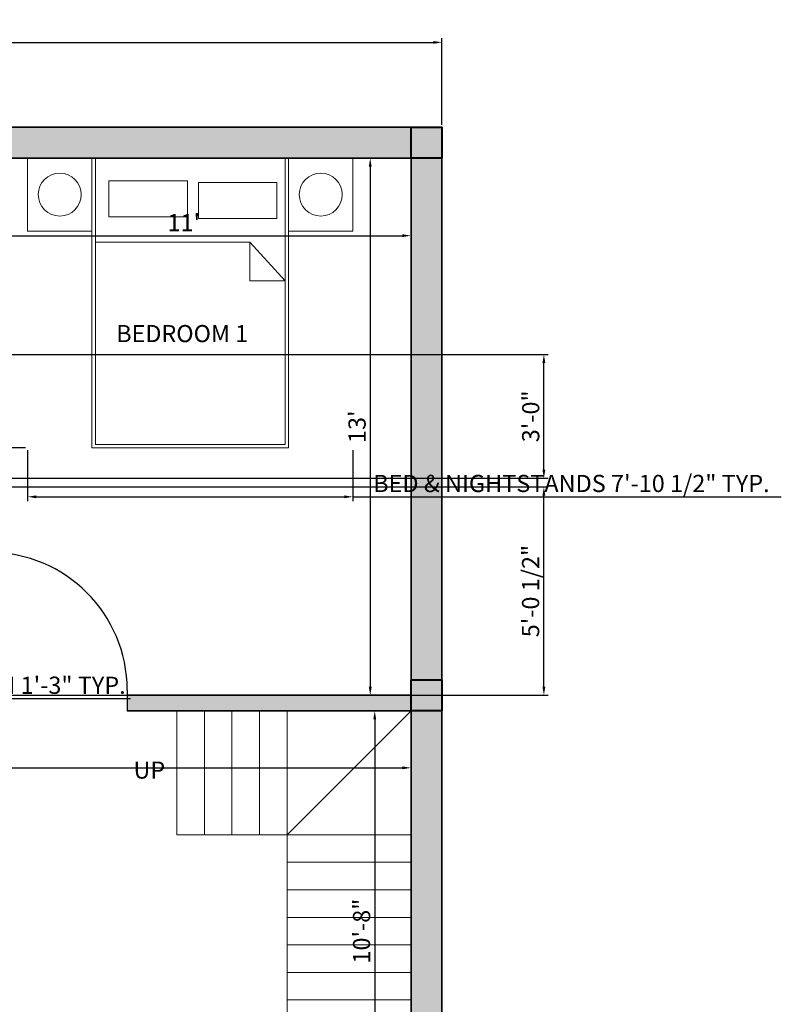
# Model space of a CAD drawing. Units: inches. Extents: x 1674 to 2231, y 1328 to 1959.
# Tile 6 of 6: x 2010 to 2231, y 1664 to 1950. Entities that reach past the tile are written whole.
import ezdxf

# ---------------------------------------------------------------- set-up
doc = ezdxf.new("R2010")
doc.units = ezdxf.units.IN
for name, color, linetype, lineweight in [('A-ANNO-DIMS', 113, 'Continuous', 18), ('A-ANNO-TEXT', 113, 'Continuous', 18), ('A-AREA-IDEN', 113, 'Continuous', 18), ('A-COLS-PATT', 10, 'Continuous', 13), ('A-FLOR-STRS', 7, 'Continuous', 18), ('A-WALL-PATT', 140, 'Continuous', 13), ('COLUMN', 10, 'Continuous', 40), ('DOOR', 54, 'Continuous', 25), ('FUR', 211, 'Continuous', 18), ('WALL', 7, 'Continuous', 35)]:
    doc.layers.add(name, color=color, linetype=linetype, lineweight=lineweight)
doc.styles.get("Standard").update_dxf_attribs({"font": 'arial.ttf'})
doc.dimstyles.new('ISO-25', dxfattribs={"dimtxt": 5, "dimasz": 2.5, "dimexe": 1.25, "dimexo": 0.625, "dimtad": 1, "dimdec": 0, "dimlunit": 4, "dimtxsty": 'Standard', "dimcen": 2.5, "dimadec": 0, "dimazin": 0, "dimtfac": 1, "dimtdec": 0, "dimtmove": 0, "dimatfit": 3, "dimfxl": 1, "dimarcsym": 0})

# ---------------------------------------------------------------- blocks, each defined once
blk = doc.blocks.new('*U2')
for p, q in [((0, 0), (0, -6)), ((40, 0), (40, -6))]:
    blk.add_line(p, q)
blk.add_lwpolyline([(0, 0), (0, 40), (1.75, 40), (1.75, 0)], close=True)
blk.add_arc((0, 0), 40, 0, 90)
blk = doc.blocks.new('*D9')
at = {"layer": 'A-ANNO-DIMS', "color": 0, "lineweight": -2, "transparency": 16777216}
for p, q in [((1736.27, 1918.98), (1736.27, 1944.21)), ((1738.77, 1942.96), (2129.77, 1942.96)), ((2132.27, 1918.98), (2132.27, 1944.21))]:
    blk.add_line(p, q, dxfattribs=at)
at = {"layer": 'A-ANNO-DIMS', "color": 0, "lineweight": 100, "transparency": 16777216}
for points in [[(1738.77, 1943.37), (1738.77, 1942.54), (1736.27, 1942.96)], [(2129.77, 1943.37), (2129.77, 1942.54), (2132.27, 1942.96)]]:
    blk.add_solid(points, dxfattribs=at)
at = {"layer": 'Defpoints', "color": 0, "lineweight": 100, "transparency": 16777216}
for p in [(2132.27, 1942.96), (1736.27, 1918.36), (2132.27, 1918.36)]:
    blk.add_point(p, dxfattribs=at)
at = {"layer": 'A-ANNO-DIMS', "color": 0, "transparency": 16777216, "insert": (1934.27, 1946.13), "char_height": 5, "attachment_point": 5}
blk.add_mtext("33'", dxfattribs=at)
blk = doc.blocks.new('*D19')
at = {"layer": 'A-ANNO-DIMS', "color": 0, "lineweight": -2, "transparency": 16777216}
for p, q in [((1991.27, 1908.73), (1991.27, 1885.57)), ((2123.27, 1908.73), (2123.27, 1885.57)), ((1993.77, 1886.82), (2120.77, 1886.82))]:
    blk.add_line(p, q, dxfattribs=at)
at = {"layer": 'A-ANNO-DIMS', "color": 0, "lineweight": 100, "transparency": 16777216}
for points in [[(1993.77, 1887.24), (1993.77, 1886.4), (1991.27, 1886.82)], [(2120.77, 1887.24), (2120.77, 1886.4), (2123.27, 1886.82)]]:
    blk.add_solid(points, dxfattribs=at)
at = {"layer": 'Defpoints', "color": 0, "lineweight": 100, "transparency": 16777216}
for p in [(1991.27, 1909.36), (2123.27, 1909.36), (2123.27, 1886.82)]:
    blk.add_point(p, dxfattribs=at)
at = {"layer": 'A-ANNO-DIMS', "color": 0, "transparency": 16777216, "insert": (2057.27, 1889.95), "char_height": 5, "attachment_point": 5}
blk.add_mtext("11'", dxfattribs=at)
blk = doc.blocks.new('*D20')
at = {"layer": 'A-ANNO-DIMS', "color": 0, "lineweight": -2, "transparency": 16777216}
for p, q in [((2122.65, 1909.36), (2110.18, 1909.36)), ((2111.43, 1906.86), (2111.43, 1755.81)), ((2122.65, 1753.31), (2110.18, 1753.31))]:
    blk.add_line(p, q, dxfattribs=at)
at = {"layer": 'A-ANNO-DIMS', "color": 0, "lineweight": 100, "transparency": 16777216}
for points in [[(2111.01, 1906.86), (2111.85, 1906.86), (2111.43, 1909.36)], [(2111.01, 1755.81), (2111.85, 1755.81), (2111.43, 1753.31)]]:
    blk.add_solid(points, dxfattribs=at)
at = {"layer": 'Defpoints', "color": 0, "lineweight": 100, "transparency": 16777216}
for p in [(2123.27, 1909.36), (2111.43, 1753.31), (2123.27, 1753.31)]:
    blk.add_point(p, dxfattribs=at)
at = {"layer": 'A-ANNO-DIMS', "color": 0, "transparency": 16777216, "insert": (2108.25, 1831.33), "char_height": 5, "attachment_point": 5, "rotation": 90}
blk.add_mtext("13'", dxfattribs=at)
blk = doc.blocks.new('*D21')
at = {"layer": 'A-ANNO-DIMS', "color": 0, "lineweight": -2, "transparency": 16777216}
for p, q in [((2122.65, 1748.86), (2111.49, 1748.86)), ((2112.74, 1746.36), (2112.74, 1623.36)), ((2122.65, 1620.86), (2111.49, 1620.86))]:
    blk.add_line(p, q, dxfattribs=at)
at = {"layer": 'A-ANNO-DIMS', "color": 0, "lineweight": 100, "transparency": 16777216}
for points in [[(2112.32, 1746.36), (2113.15, 1746.36), (2112.74, 1748.86)], [(2112.32, 1623.36), (2113.15, 1623.36), (2112.74, 1620.86)]]:
    blk.add_solid(points, dxfattribs=at)
at = {"layer": 'Defpoints', "color": 0, "lineweight": 100, "transparency": 16777216}
for p in [(2123.27, 1748.86), (2112.74, 1620.86), (2123.27, 1620.86)]:
    blk.add_point(p, dxfattribs=at)
at = {"layer": 'A-ANNO-DIMS', "color": 0, "transparency": 16777216, "insert": (2109.56, 1684.86), "char_height": 5, "attachment_point": 5, "rotation": 90}
blk.add_mtext('10\'-8"', dxfattribs=at)
blk = doc.blocks.new('*D33')
at = {"layer": 'A-ANNO-DIMS', "color": 0, "lineweight": -2, "transparency": 16777216}
for p, q in [((1821.77, 1748.23), (1821.77, 1731.03)), ((2123.27, 1748.18), (2123.27, 1731.03)), ((1824.27, 1732.28), (2120.77, 1732.28))]:
    blk.add_line(p, q, dxfattribs=at)
at = {"layer": 'A-ANNO-DIMS', "color": 0, "lineweight": 100, "transparency": 16777216}
for points in [[(1824.27, 1732.69), (1824.27, 1731.86), (1821.77, 1732.28)], [(2120.77, 1732.69), (2120.77, 1731.86), (2123.27, 1732.28)]]:
    blk.add_solid(points, dxfattribs=at)
at = {"layer": 'Defpoints', "color": 0, "lineweight": 100, "transparency": 16777216}
for p in [(1821.77, 1748.86), (2123.27, 1748.81), (2123.27, 1732.28)]:
    blk.add_point(p, dxfattribs=at)
at = {"layer": 'A-ANNO-DIMS', "color": 0, "transparency": 16777216, "insert": (1972.52, 1735.45), "char_height": 5, "attachment_point": 5}
blk.add_mtext('25\'-2"', dxfattribs=at)
blk = doc.blocks.new('BED-DOUBLE-WITH-NIGHTSTANDS')
for p, q in [((35.61, 74.81), (24.38, 64.59)), ((35.61, 64.59), (35.61, 74.81)), ((24.38, 19.67), (24.38, 64.59)), ((24.38, 64.59), (35.61, 64.59))]:
    blk.add_line(p, q)
for points in [[(0, 75.81), (21.22, 75.81), (21.22, 94.48), (0, 94.48)], [(0, 19.67), (83.2, 19.67), (83.2, 74.81), (0, 74.81)], [(7.05, 49.62), (17.52, 49.62), (17.52, 72.41), (7.05, 72.41)], [(6.58, 23.6), (17.06, 23.6), (17.06, 46.39), (6.58, 46.39)], [(0, 0), (21.22, 0), (21.22, 18.67), (0, 18.67)]]:
    blk.add_lwpolyline(points, close=True)
blk.add_lwpolyline([(0, 18.67), (84.2, 18.67), (84.2, 75.81), (0, 75.81)])
for centre in [(10.61, 85.15), (10.61, 9.33)]:
    blk.add_circle(centre, 6.24)
blk = doc.blocks.new('*D42')
at = {"layer": 'A-ANNO-DIMS', "color": 0, "lineweight": -2, "transparency": 16777216}
for p, q in [((1969.88, 1754.02), (1969.88, 1751.15)), ((1984.85, 1754.02), (1984.85, 1751.15)), ((1972.38, 1752.4), (1982.35, 1752.4)), ((1984.85, 1752.4), (2041.76, 1752.4))]:
    blk.add_line(p, q, dxfattribs=at)
at = {"layer": 'A-ANNO-DIMS', "color": 0, "lineweight": 100, "transparency": 16777216}
for points in [[(1972.38, 1752.81), (1972.38, 1751.98), (1969.88, 1752.4)], [(1982.35, 1752.81), (1982.35, 1751.98), (1984.85, 1752.4)]]:
    blk.add_solid(points, dxfattribs=at)
at = {"layer": 'Defpoints', "color": 0, "lineweight": 100, "transparency": 16777216}
for p in [(1969.88, 1754.64), (1984.85, 1754.64), (1984.85, 1752.4)]:
    blk.add_point(p, dxfattribs=at)
at = {"layer": 'A-ANNO-DIMS', "color": 0, "transparency": 16777216, "insert": (2014.56, 1755.61), "char_height": 5, "attachment_point": 5}
blk.add_mtext('BASIN 1\'-3" TYP.', dxfattribs=at)
blk = doc.blocks.new('*D46')
at = {"layer": 'A-ANNO-DIMS', "color": 0, "lineweight": -2, "transparency": 16777216}
for p, q in [((2011.91, 1824.53), (2011.91, 1809.74)), ((2106.39, 1824.53), (2106.39, 1809.74)), ((2014.41, 1810.99), (2103.89, 1810.99)), ((2106.39, 1810.99), (2230.84, 1810.99))]:
    blk.add_line(p, q, dxfattribs=at)
at = {"layer": 'A-ANNO-DIMS', "color": 0, "lineweight": 100, "transparency": 16777216}
for points in [[(2014.41, 1811.4), (2014.41, 1810.57), (2011.91, 1810.99)], [(2103.89, 1811.4), (2103.89, 1810.57), (2106.39, 1810.99)]]:
    blk.add_solid(points, dxfattribs=at)
at = {"layer": 'Defpoints', "color": 0, "lineweight": 100, "transparency": 16777216}
for p in [(2011.91, 1825.16), (2106.39, 1825.16), (2106.39, 1810.99)]:
    blk.add_point(p, dxfattribs=at)
at = {"layer": 'A-ANNO-DIMS', "color": 0, "transparency": 16777216, "insert": (2169.86, 1814.21), "char_height": 5, "attachment_point": 5}
blk.add_mtext('BED & NIGHTSTANDS 7\'-10 1/2" TYP.', dxfattribs=at)
blk = doc.blocks.new('*D47')
at = {"layer": 'A-ANNO-DIMS', "color": 0, "lineweight": -2, "transparency": 16777216}
for p, q in [((2011.29, 1909.36), (1996.49, 1909.36)), ((1997.74, 1906.86), (1997.74, 1827.66)), ((2011.29, 1825.16), (1996.49, 1825.16))]:
    blk.add_line(p, q, dxfattribs=at)
at = {"layer": 'A-ANNO-DIMS', "color": 0, "lineweight": 100, "transparency": 16777216}
for points in [[(1997.32, 1906.86), (1998.16, 1906.86), (1997.74, 1909.36)], [(1997.32, 1827.66), (1998.16, 1827.66), (1997.74, 1825.16)]]:
    blk.add_solid(points, dxfattribs=at)
at = {"layer": 'Defpoints', "color": 0, "lineweight": 100, "transparency": 16777216}
for p in [(2011.91, 1909.36), (1997.74, 1825.16), (2011.91, 1825.16)]:
    blk.add_point(p, dxfattribs=at)
at = {"layer": 'A-ANNO-DIMS', "color": 0, "transparency": 16777216, "insert": (1994.56, 1867.26), "char_height": 5, "attachment_point": 5, "rotation": 90}
blk.add_mtext('7\'-0" TYP.', dxfattribs=at)
blk = doc.blocks.new('*D52')
at = {"layer": 'A-ANNO-DIMS', "color": 0, "lineweight": -2, "transparency": 16777216}
for p, q in [((1987.4, 1813.86), (2163.12, 1813.86)), ((2161.87, 1755.86), (2161.87, 1811.36)), ((1987.4, 1753.36), (2163.12, 1753.36))]:
    blk.add_line(p, q, dxfattribs=at)
at = {"layer": 'A-ANNO-DIMS', "color": 0, "lineweight": 100, "transparency": 16777216}
for points in [[(2161.45, 1811.36), (2162.29, 1811.36), (2161.87, 1813.86)], [(2161.45, 1755.86), (2162.29, 1755.86), (2161.87, 1753.36)]]:
    blk.add_solid(points, dxfattribs=at)
at = {"layer": 'Defpoints', "color": 0, "lineweight": 100, "transparency": 16777216}
for p in [(1986.77, 1813.86), (2161.87, 1813.86), (1986.77, 1753.36)]:
    blk.add_point(p, dxfattribs=at)
at = {"layer": 'A-ANNO-DIMS', "color": 0, "transparency": 16777216, "insert": (2158.66, 1783.61), "char_height": 5, "attachment_point": 5, "rotation": 90}
blk.add_mtext('5\'-0 1/2"', dxfattribs=at)
blk = doc.blocks.new('*D53')
at = {"layer": 'A-ANNO-DIMS', "color": 0, "lineweight": -2, "transparency": 16777216}
for p, q in [((1987.4, 1852.36), (2163.12, 1852.36)), ((2161.87, 1818.86), (2161.87, 1849.86)), ((1987.4, 1816.36), (2163.12, 1816.36))]:
    blk.add_line(p, q, dxfattribs=at)
at = {"layer": 'A-ANNO-DIMS', "color": 0, "lineweight": 100, "transparency": 16777216}
for points in [[(2161.45, 1849.86), (2162.29, 1849.86), (2161.87, 1852.36)], [(2161.45, 1818.86), (2162.29, 1818.86), (2161.87, 1816.36)]]:
    blk.add_solid(points, dxfattribs=at)
at = {"layer": 'Defpoints', "color": 0, "lineweight": 100, "transparency": 16777216}
for p in [(1986.77, 1852.36), (2161.87, 1852.36), (1986.77, 1816.36)]:
    blk.add_point(p, dxfattribs=at)
at = {"layer": 'A-ANNO-DIMS', "color": 0, "transparency": 16777216, "insert": (2158.69, 1834.36), "char_height": 5, "attachment_point": 5, "rotation": 90}
blk.add_mtext('3\'-0"', dxfattribs=at)

msp = doc.modelspace()

# ---------------------------------------------------------------- hatches: boundary and pattern name
at = {"layer": 'A-COLS-PATT'}
h = msp.add_hatch(color=256, dxfattribs=at)
h.dxf.hatch_style = 1
h.paths.add_polyline_path([(1745.27, 1918.36), (1736.27, 1918.36), (1736.27, 1909.36), (1745.27, 1909.36)])
h.paths.add_polyline_path([(1886.27, 1918.36), (1877.27, 1918.36), (1877.27, 1909.36), (1886.27, 1909.36)])
h.paths.add_polyline_path([(1995.77, 1918.36), (1986.77, 1918.36), (1986.77, 1909.36), (1995.77, 1909.36)])
h.paths.add_polyline_path([(2132.27, 1918.36), (2123.27, 1918.36), (2123.27, 1909.36), (2132.27, 1909.36)])
h.paths.add_polyline_path([(1745.27, 1757.86), (1736.27, 1757.86), (1736.27, 1748.86), (1745.27, 1748.86)])
h.paths.add_polyline_path([(1886.27, 1757.86), (1877.27, 1757.86), (1877.27, 1748.86), (1886.27, 1748.86)])
h.paths.add_polyline_path([(2132.27, 1757.81), (2123.27, 1757.81), (2123.27, 1748.81), (2132.27, 1748.81)])
h.paths.add_polyline_path([(1995.77, 1757.86), (1986.77, 1757.86), (1986.77, 1748.86), (1995.77, 1748.86)])
h.paths.add_polyline_path([(2132.27, 1625.36), (2123.27, 1625.36), (2123.27, 1616.36), (2132.27, 1616.36)])
h.paths.add_polyline_path([(1995.77, 1625.36), (1986.77, 1625.36), (1986.77, 1616.36), (1995.77, 1616.36)])
h.paths.add_polyline_path([(1869.77, 1604.86), (1860.77, 1604.86), (1860.77, 1595.86), (1869.77, 1595.86)])
h.paths.add_polyline_path([(1745.27, 1609.36), (1736.27, 1609.36), (1736.27, 1600.36), (1745.27, 1600.36)])
h.paths.add_polyline_path([(1745.27, 1504.36), (1736.27, 1504.36), (1736.27, 1495.36), (1745.27, 1495.36)])
h.paths.add_polyline_path([(1870.95, 1504.36), (1861.95, 1504.36), (1861.95, 1495.36), (1870.95, 1495.36)])
h.paths.add_polyline_path([(1995.77, 1504.36), (1986.77, 1504.36), (1986.77, 1495.36), (1995.77, 1495.36)])
h.paths.add_polyline_path([(1995.77, 1447.36), (1986.77, 1447.36), (1986.77, 1438.36), (1995.77, 1438.36)])
h.paths.add_polyline_path([(2132.27, 1447.36), (2123.27, 1447.36), (2123.27, 1438.36), (2132.27, 1438.36)])
at = {"layer": 'A-WALL-PATT'}
h = msp.add_hatch(color=256, dxfattribs=at)
h.dxf.hatch_style = 1
h.paths.add_polyline_path([(1877.27, 1918.36), (1745.27, 1918.36), (1745.27, 1909.36), (1877.27, 1909.36)])
h.paths.add_polyline_path([(1986.77, 1918.36), (1886.27, 1918.36), (1886.27, 1909.36), (1986.77, 1909.36)])
h.paths.add_polyline_path([(2123.27, 1918.36), (1995.77, 1918.36), (1995.77, 1909.36), (2123.27, 1909.36)])
h.paths.add_polyline_path([(1894.11, 1861.36), (1886.27, 1861.36), (1886.27, 1865.74), (1881.77, 1865.74), (1881.77, 1808), (1881.77, 1798.89), (1884.87, 1798.89, -0.017002), (1886.27, 1798.84), (1886.27, 1852.36), (1894.11, 1852.36)])
h.paths.add_polyline_path([(1952.87, 1861.36), (1919.24, 1861.36), (1919.24, 1852.36), (1952.87, 1852.36)])
h.paths.add_polyline_path([(1991.27, 1865.74), (1986.77, 1865.74), (1986.77, 1861.36), (1976.26, 1861.36), (1976.26, 1852.36), (1986.77, 1852.36), (1986.77, 1847.49), (1986.77, 1757.86), (1991.27, 1757.86), (1991.27, 1852.36)])
h.paths.add_polyline_path([(1986.77, 1816.36), (1938.77, 1816.36), (1938.77, 1813.86), (1986.77, 1813.86)])
h.paths.add_polyline_path([(1934.27, 1819.36), (1886.27, 1819.36), (1886.27, 1816.86), (1934.27, 1816.86)])
h.paths.add_polyline_path([(1938.77, 1852.36), (1934.27, 1852.36), (1934.27, 1753.36), (1934.27, 1748.86), (1938.77, 1748.86), (1938.77, 1753.36)])
h.paths.add_polyline_path([(1934.27, 1777.36), (1915.46, 1777.36), (1886.27, 1777.36), (1886.27, 1772.86), (1934.27, 1772.86)])
h.paths.add_polyline_path([(1986.77, 1753.36), (1967.96, 1753.36), (1961.77, 1753.36, -0.017002), (1961.81, 1751.95), (1961.81, 1748.86), (1986.77, 1748.86)])
h.paths.add_polyline_path([(2000.84, 1753.36), (1995.77, 1753.36), (1995.77, 1748.86), (2000.84, 1748.86)])
h.paths.add_polyline_path([(1941.17, 1751.95), (1941.17, 1753.36), (1938.77, 1753.36), (1938.77, 1748.86), (1941.17, 1748.86)])
h.paths.add_polyline_path([(1877.27, 1753.36), (1875.49, 1753.36), (1875.49, 1748.86), (1877.27, 1748.86)])
h.paths.add_polyline_path([(1745.27, 1909.36), (1736.27, 1909.36), (1736.27, 1757.86), (1745.27, 1757.86), (1745.27, 1773.01)])
h.paths.add_polyline_path([(1778.41, 1645.36), (1745.27, 1645.36), (1745.27, 1640.86), (1778.41, 1640.86)])
h.paths.add_polyline_path([(1821.77, 1645.36), (1821.77, 1668.45), (1817.27, 1668.45), (1817.27, 1645.36), (1817.27, 1640.86), (1821.77, 1640.86)])
h.paths.add_polyline_path([(1817.27, 1645.36), (1813.39, 1645.36), (1813.39, 1640.86), (1817.27, 1640.86)])
h.paths.add_polyline_path([(1821.77, 1640.86), (1817.27, 1640.86), (1817.27, 1604.86), (1817.27, 1600.36), (1821.77, 1600.36)])
h.paths.add_polyline_path([(1825.14, 1604.86), (1821.77, 1604.86), (1821.77, 1600.36), (1825.14, 1600.36)])
h.paths.add_polyline_path([(1781.27, 1604.86), (1745.27, 1604.86), (1745.27, 1600.36), (1781.27, 1600.36)])
h = msp.add_hatch(color=256, dxfattribs=at)
h.dxf.hatch_style = 1
h.paths.add_polyline_path([(2132.27, 1909.36), (2123.27, 1909.36), (2123.27, 1757.81), (2132.27, 1757.81)], flags=17)
h.paths.add_polyline_path([(2123.27, 1753.36), (2040.84, 1753.36), (2040.84, 1748.86), (2123.27, 1748.86)], flags=17)
h.paths.add_polyline_path([(1840.51, 1753.36), (1745.27, 1753.36), (1745.27, 1748.86), (1817.27, 1748.86), (1840.51, 1748.86)], flags=17)
h.paths.add_polyline_path([(1745.27, 1748.86), (1736.27, 1748.86), (1736.27, 1609.36), (1745.27, 1609.36), (1745.27, 1640.86)], flags=17)
h.paths.add_polyline_path([(1745.27, 1600.36), (1736.27, 1600.36), (1736.27, 1504.36), (1745.27, 1504.36)], flags=17)
h.paths.add_polyline_path([(1745.27, 1495.36), (1736.27, 1495.36), (1736.27, 1447.36), (1745.27, 1447.36)], flags=17)
h.paths.add_polyline_path([(1820.35, 1504.36), (1787.69, 1504.36), (1787.69, 1495.36), (1820.35, 1495.36)], flags=17)
h.paths.add_polyline_path([(1750.58, 1504.36), (1745.27, 1504.36), (1745.27, 1495.36), (1750.58, 1495.36)], flags=17)
h.paths.add_polyline_path([(1861.95, 1504.36), (1857.47, 1504.36), (1857.47, 1495.36), (1861.95, 1495.36)], flags=17)
h.paths.add_polyline_path([(1873.66, 1504.36), (1870.95, 1504.36), (1870.95, 1495.36), (1873.66, 1495.36)], flags=17)
h.paths.add_polyline_path([(1900.85, 1501.36), (1900.85, 1504.36), (1895.88, 1504.36), (1895.88, 1495.36), (1900.85, 1495.36)], flags=17)
h.paths.add_polyline_path([(1869.77, 1595.86), (1865.27, 1595.86), (1865.27, 1504.36), (1869.77, 1504.36)], flags=17)
h.paths.add_polyline_path([(1958.26, 1504.36), (1940.74, 1504.36, -0.01877), (1940.85, 1501.36), (1940.85, 1495.36), (1958.26, 1495.36)], flags=17)
h.paths.add_polyline_path([(1995.77, 1531.51), (1986.77, 1531.51), (1986.77, 1504.36), (1995.77, 1504.36)], flags=17)
h.paths.add_polyline_path([(1986.77, 1504.36), (1980.49, 1504.36), (1980.49, 1495.36), (1986.77, 1495.36)], flags=17)
h.paths.add_polyline_path([(1995.77, 1616.36), (1986.77, 1616.36), (1986.77, 1585.02), (1995.77, 1585.02)], flags=17)
h.paths.add_polyline_path([(2000.1, 1620.86), (1995.77, 1620.86), (1995.77, 1616.36), (2000.1, 1616.36)], flags=17)
h.paths.add_polyline_path([(2053.57, 1620.86), (2040.1, 1620.86), (2040.1, 1616.36), (2053.57, 1616.36)], flags=17)
h.paths.add_polyline_path([(2123.27, 1620.86), (2109.12, 1620.86), (2109.12, 1616.36), (2123.27, 1616.36)], flags=17)
h.paths.add_polyline_path([(2132.27, 1616.36), (2123.27, 1616.36), (2123.27, 1447.36), (2132.27, 1447.36)], flags=17)
h.paths.add_polyline_path([(1986.77, 1447.36), (1870.95, 1447.36), (1870.95, 1438.36), (1986.77, 1438.36)])
h.paths.add_polyline_path([(1861.95, 1447.36), (1745.27, 1447.36), (1745.27, 1438.36), (1861.95, 1438.36)])
h.paths.add_polyline_path([(2132.27, 1918.36), (1736.27, 1918.36), (1736.27, 1504.36), (1745.27, 1504.36), (1745.27, 1600.36), (1745.27, 1909.36), (2123.27, 1909.36), (2123.27, 1447.36), (2132.27, 1447.36)])
h = msp.add_hatch(color=256, dxfattribs=at)
h.dxf.hatch_style = 1
h.paths.add_polyline_path([(1886.27, 1777.36), (1886.27, 1778.24), (1884.87, 1778.24), (1881.77, 1778.24), (1881.77, 1757.86), (1886.27, 1757.86)], flags=17)
h.paths.add_polyline_path([(2132.27, 1918.36), (1736.27, 1918.36), (1736.27, 1757.86), (1745.27, 1757.86), (1745.27, 1773.01), (1745.27, 1909.36), (2123.27, 1909.36), (2123.27, 1757.81), (2132.27, 1757.81)])

# ---------------------------------------------------------------- linework, layer by layer
at = {"layer": 'A-FLOR-STRS'}
for p, q in [((2055.27, 1712.86), (2055.27, 1748.86)), ((2063.27, 1712.86), (2063.27, 1748.86)), ((2071.27, 1712.86), (2071.27, 1748.86)), ((2079.27, 1712.86), (2079.27, 1748.86)), ((2087.27, 1712.86), (2087.27, 1748.86)), ((2123.27, 1748.81), (2087.27, 1712.86)), ((2087.27, 1712.86), (2055.27, 1712.86)), ((2087.27, 1656.86), (2087.27, 1712.86)), ((2087.27, 1712.86), (2123.27, 1712.86)), ((2087.27, 1704.86), (2123.27, 1704.86)), ((2087.27, 1696.86), (2123.27, 1696.86)), ((2087.27, 1688.86), (2123.27, 1688.86)), ((2087.27, 1680.86), (2123.27, 1680.86)), ((2087.27, 1672.86), (2123.27, 1672.86)), ((2087.27, 1664.86), (2123.27, 1664.86))]:
    msp.add_line(p, q, dxfattribs=at)
at = {"layer": 'COLUMN'}
for points in [[(2123.27, 1918.36), (2132.27, 1918.36), (2132.27, 1909.36), (2123.27, 1909.36)], [(2123.27, 1757.81), (2132.27, 1757.81), (2132.27, 1748.81), (2123.27, 1748.81)]]:
    msp.add_lwpolyline(points, close=True, dxfattribs=at)
at = {"layer": 'WALL'}
for p, q in [((1736.27, 1918.36), (2132.27, 1918.36)), ((2132.27, 1918.36), (2132.27, 1438.36)), ((2040.84, 1753.36), (2123.27, 1753.36)), ((2040.84, 1748.86), (2123.27, 1748.86))]:
    msp.add_line(p, q, dxfattribs=at)
for points in [[(1995.77, 1438.36), (1736.27, 1438.36), (1736.27, 1918.36), (2132.27, 1918.36), (2132.27, 1438.36), (2123.27, 1438.36)], [(1995.77, 1447.36), (1745.27, 1447.36), (1745.27, 1909.36), (2123.27, 1909.36), (2123.27, 1447.36)]]:
    msp.add_lwpolyline(points, dxfattribs=at)

# ---------------------------------------------------------------- block references
at = {"layer": 'DOOR'}
msp.add_blockref('*U2', (2000.84, 1754.86), dxfattribs=at)
at = {"layer": 'FUR', "rotation": 270.0000000000002}
msp.add_blockref('BED-DOUBLE-WITH-NIGHTSTANDS', (2011.91, 1909.36), dxfattribs=at)

# ---------------------------------------------------------------- texts
at = {"layer": 'A-ANNO-TEXT', "insert": (2042.66, 1734.11), "char_height": 4.973, "attachment_point": 1}
msp.add_mtext_dynamic_manual_height_columns('UP', width=89.7127, gutter_width=24.87, heights=[0], dxfattribs=at)
at = {"layer": 'A-AREA-IDEN', "insert": (2037.66, 1860.87), "char_height": 4.973, "attachment_point": 1}
msp.add_mtext_dynamic_manual_height_columns('BEDROOM 1', width=89.7127, gutter_width=24.87, heights=[0], dxfattribs=at)

# ---------------------------------------------------------------- dimensions: what is measured, and where the dimension line sits
at = {"layer": 'A-ANNO-DIMS'}
for base, p1, p2, picture, middle in [((2132.27, 1942.96), (1736.27, 1918.36), (2132.27, 1918.36), '*D9', (1934.27, 1946.13)), ((2123.27, 1886.82), (1991.27, 1909.36), (2123.27, 1909.36), '*D19', (2057.27, 1889.95)), ((2123.27109151, 1732.2761534), (1821.77109151, 1748.85548105), (2123.27109151, 1748.80863988), '*D33', (1972.52109151, 1735.45401834))]:
    dim = msp.add_linear_dim(base=base, p1=p1, p2=p2, dimstyle='ISO-25', override={"dimclrd": 0, "dimclre": 0, "dimclrt": 0}, dxfattribs=at)
    dim.commit()
    dim.dimension.update_dxf_attribs({"geometry": picture, "text_midpoint": middle})
for base, p1, p2, angle, text, picture, middle in [((1997.74, 1825.16), (2011.91, 1909.36), (2011.91, 1825.16), 270, '<> TYP.', '*D47', (1994.56, 1867.26)), ((2106.39, 1810.99), (2011.91, 1825.16), (2106.39, 1825.16), 0, 'BED & NIGHTSTANDS <> TYP.', '*D46', (2169.86, 1814.21))]:
    dim = msp.add_linear_dim(base=base, p1=p1, p2=p2, angle=angle, text=text, dimstyle='ISO-25', override={"dimdec": 1, "dimlfac": 1, "dimrnd": 0, "dimzin": 1, "dimdsep": 46, "dimlunit": 4, "dimfrac": 2}, dxfattribs=at)
    dim.commit()
    dim.dimension.update_dxf_attribs({"geometry": picture, "text_midpoint": middle})
for base, p1, p2, override, picture, middle in [((2111.43, 1753.31), (2123.27, 1909.36), (2123.27, 1753.31), {"dimclrd": 0, "dimclre": 0, "dimclrt": 0}, '*D20', (2108.25, 1831.33)), ((2161.87, 1852.36), (1986.77, 1816.36), (1986.77, 1852.36), {"dimdec": 1, "dimlfac": 1, "dimrnd": 0, "dimzin": 1, "dimdsep": 46, "dimlunit": 4, "dimfrac": 2}, '*D53', (2158.69, 1834.36)), ((2161.87, 1813.86), (1986.77, 1753.36), (1986.77, 1813.86), {"dimdec": 1, "dimlfac": 1, "dimrnd": 0, "dimzin": 1, "dimdsep": 46, "dimlunit": 4, "dimfrac": 2}, '*D52', (2158.66, 1783.61)), ((2112.74, 1620.86), (2123.27, 1748.86), (2123.27, 1620.86), {"dimclrd": 0, "dimclre": 0, "dimclrt": 0}, '*D21', (2109.56, 1684.86))]:
    dim = msp.add_linear_dim(base=base, p1=p1, p2=p2, angle=90, dimstyle='ISO-25', override=override, dxfattribs=at)
    dim.commit()
    dim.dimension.update_dxf_attribs({"geometry": picture, "text_midpoint": middle})
dim = msp.add_linear_dim(base=(1984.85, 1752.4), p1=(1969.88, 1754.64), p2=(1984.85, 1754.64), text='BASIN <> TYP.', dimstyle='ISO-25', override={"dimdec": 1, "dimlfac": 1, "dimrnd": 0, "dimzin": 1, "dimdsep": 46, "dimlunit": 4, "dimfrac": 2}, dxfattribs=at)
dim.commit()
dim.dimension.update_dxf_attribs({"geometry": '*D42', "text_midpoint": (2014.56, 1755.61)})

doc.saveas('drawing.dxf')
